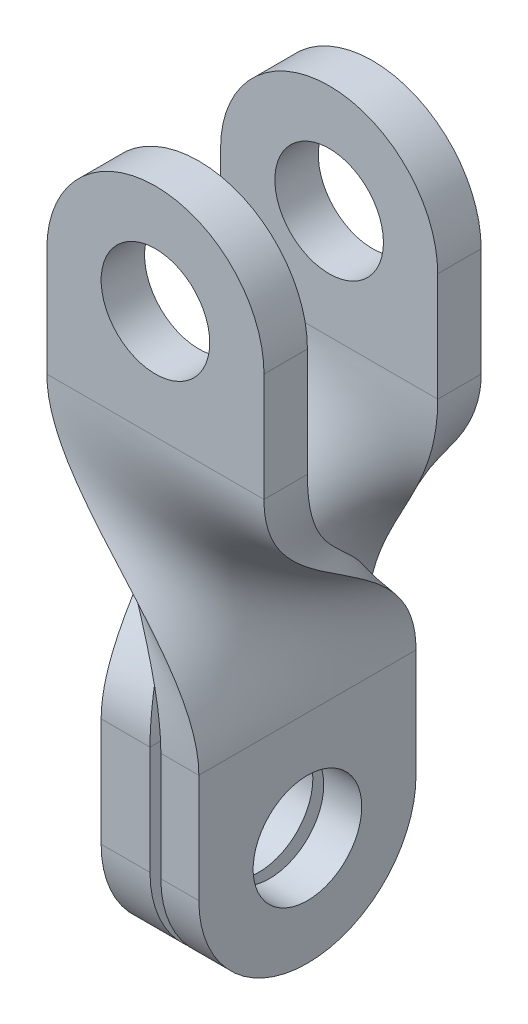
ISO-10303-21;
HEADER;
FILE_DESCRIPTION(('STEP AP214'),'2;1');
FILE_NAME('part.step','',(''),(''),'','','');
FILE_SCHEMA(('AUTOMOTIVE_DESIGN { 1 0 10303 214 1 1 1 1 }'));
ENDSEC;
DATA;
#1=APPLICATION_CONTEXT('core data for automotive mechanical design processes');
#2=APPLICATION_PROTOCOL_DEFINITION('international standard','automotive_design',2000,#1);
#3=PRODUCT_CONTEXT('',#1,'mechanical');
#4=PRODUCT('Part','Part','',(#3));
#5=PRODUCT_RELATED_PRODUCT_CATEGORY('part','',(#4));
#6=PRODUCT_DEFINITION_FORMATION('','',#4);
#7=PRODUCT_DEFINITION_CONTEXT('part definition',#1,'design');
#8=PRODUCT_DEFINITION('design','',#6,#7);
#9=PRODUCT_DEFINITION_SHAPE('','',#8);
#10=(LENGTH_UNIT() NAMED_UNIT(*) SI_UNIT(.MILLI.,.METRE.));
#11=(NAMED_UNIT(*) PLANE_ANGLE_UNIT() SI_UNIT($,.RADIAN.));
#12=(NAMED_UNIT(*) SI_UNIT($,.STERADIAN.) SOLID_ANGLE_UNIT());
#13=UNCERTAINTY_MEASURE_WITH_UNIT(LENGTH_MEASURE(1.E-05),#10,'distance_accuracy_value','');
#14=(GEOMETRIC_REPRESENTATION_CONTEXT(3) GLOBAL_UNCERTAINTY_ASSIGNED_CONTEXT((#13)) GLOBAL_UNIT_ASSIGNED_CONTEXT((#10,
#11,#12)) REPRESENTATION_CONTEXT('',''));
#15=CARTESIAN_POINT('',(0.,0.,0.));
#16=DIRECTION('',(0.,0.,1.));
#17=DIRECTION('',(1.,0.,0.));
#18=AXIS2_PLACEMENT_3D('',#15,#16,#17);
#19=CARTESIAN_POINT('',(-0.5,-4.5,1.));
#20=DIRECTION('',(0.,0.,-1.));
#21=DIRECTION('',(-1.,0.,0.));
#22=AXIS2_PLACEMENT_3D('',#19,#20,#21);
#23=PLANE('',#22);
#24=DIRECTION('',(0.,-1.,0.));
#25=VECTOR('',#24,1.);
#26=CARTESIAN_POINT('',(-0.05,-4.5,1.));
#27=LINE('',#26,#25);
#28=CARTESIAN_POINT('',(-0.05,-3.5,1.));
#29=VERTEX_POINT('',#28);
#30=CARTESIAN_POINT('',(-0.05,-4.5,1.));
#31=VERTEX_POINT('',#30);
#32=EDGE_CURVE('E577',#29,#31,#27,.T.);
#33=ORIENTED_EDGE('',*,*,#32,.F.);
#34=DIRECTION('',(1.,0.,0.));
#35=VECTOR('',#34,1.);
#36=CARTESIAN_POINT('',(-0.5,-3.5,1.));
#37=LINE('',#36,#35);
#38=CARTESIAN_POINT('',(-0.5,-3.5,1.));
#39=VERTEX_POINT('',#38);
#40=EDGE_CURVE('E604',#39,#29,#37,.T.);
#41=ORIENTED_EDGE('',*,*,#40,.F.);
#42=DIRECTION('',(0.,1.,0.));
#43=VECTOR('',#42,1.);
#44=CARTESIAN_POINT('',(-0.5,-4.5,1.));
#45=LINE('',#44,#43);
#46=CARTESIAN_POINT('',(-0.5,-4.5,1.));
#47=VERTEX_POINT('',#46);
#48=EDGE_CURVE('E598',#47,#39,#45,.T.);
#49=ORIENTED_EDGE('',*,*,#48,.F.);
#50=DIRECTION('',(1.,0.,0.));
#51=VECTOR('',#50,1.);
#52=CARTESIAN_POINT('',(-0.5,-4.5,1.));
#53=LINE('',#52,#51);
#54=EDGE_CURVE('E546',#47,#31,#53,.T.);
#55=ORIENTED_EDGE('',*,*,#54,.T.);
#56=EDGE_LOOP('',(#33,#41,#49,#55));
#57=FACE_BOUND('',#56,.T.);
#58=ADVANCED_FACE('F544',(#57),#23,.F.);
#59=CARTESIAN_POINT('',(-0.5,-3.5,1.));
#60=DIRECTION('',(0.,-1.,0.));
#61=DIRECTION('',(0.,0.,-1.));
#62=AXIS2_PLACEMENT_3D('',#59,#60,#61);
#63=PLANE('',#62);
#64=DIRECTION('',(0.,0.,1.));
#65=VECTOR('',#64,1.);
#66=CARTESIAN_POINT('',(-0.05,-3.5,1.));
#67=LINE('',#66,#65);
#68=CARTESIAN_POINT('',(-0.05,-3.5,-1.));
#69=VERTEX_POINT('',#68);
#70=EDGE_CURVE('E14',#69,#29,#67,.T.);
#71=ORIENTED_EDGE('',*,*,#70,.F.);
#72=DIRECTION('',(1.,0.,0.));
#73=VECTOR('',#72,1.);
#74=CARTESIAN_POINT('',(-0.5,-3.5,-1.));
#75=LINE('',#74,#73);
#76=CARTESIAN_POINT('',(-0.5,-3.5,-1.));
#77=VERTEX_POINT('',#76);
#78=EDGE_CURVE('E593',#77,#69,#75,.T.);
#79=ORIENTED_EDGE('',*,*,#78,.F.);
#80=DIRECTION('',(0.,0.,-1.));
#81=VECTOR('',#80,1.);
#82=CARTESIAN_POINT('',(-0.5,-3.5,1.));
#83=LINE('',#82,#81);
#84=EDGE_CURVE('E614',#39,#77,#83,.T.);
#85=ORIENTED_EDGE('',*,*,#84,.F.);
#86=ORIENTED_EDGE('',*,*,#40,.T.);
#87=EDGE_LOOP('',(#71,#79,#85,#86));
#88=FACE_BOUND('',#87,.T.);
#89=ADVANCED_FACE('F621',(#88),#63,.F.);
#90=CARTESIAN_POINT('',(-0.5,-3.5,-1.));
#91=DIRECTION('',(0.,0.,1.));
#92=DIRECTION('',(0.,-1.,0.));
#93=AXIS2_PLACEMENT_3D('',#90,#91,#92);
#94=PLANE('',#93);
#95=DIRECTION('',(0.,1.,0.));
#96=VECTOR('',#95,1.);
#97=CARTESIAN_POINT('',(-0.05,-3.5,-1.));
#98=LINE('',#97,#96);
#99=CARTESIAN_POINT('',(-0.05,-4.5,-1.));
#100=VERTEX_POINT('',#99);
#101=EDGE_CURVE('E552',#100,#69,#98,.T.);
#102=ORIENTED_EDGE('',*,*,#101,.F.);
#103=DIRECTION('',(1.,0.,0.));
#104=VECTOR('',#103,1.);
#105=CARTESIAN_POINT('',(-0.5,-4.5,-1.));
#106=LINE('',#105,#104);
#107=CARTESIAN_POINT('',(-0.5,-4.5,-1.));
#108=VERTEX_POINT('',#107);
#109=EDGE_CURVE('E591',#108,#100,#106,.T.);
#110=ORIENTED_EDGE('',*,*,#109,.F.);
#111=DIRECTION('',(0.,-1.,0.));
#112=VECTOR('',#111,1.);
#113=CARTESIAN_POINT('',(-0.5,-3.5,-1.));
#114=LINE('',#113,#112);
#115=EDGE_CURVE('E615',#77,#108,#114,.T.);
#116=ORIENTED_EDGE('',*,*,#115,.F.);
#117=ORIENTED_EDGE('',*,*,#78,.T.);
#118=EDGE_LOOP('',(#102,#110,#116,#117));
#119=FACE_BOUND('',#118,.T.);
#120=ADVANCED_FACE('F586',(#119),#94,.F.);
#121=CARTESIAN_POINT('',(-0.5,-4.5,0.));
#122=DIRECTION('',(1.,0.,0.));
#123=DIRECTION('',(0.,0.,-1.));
#124=AXIS2_PLACEMENT_3D('',#121,#122,#123);
#125=CYLINDRICAL_SURFACE('',#124,1.);
#126=CARTESIAN_POINT('',(-0.05,-4.5,0.));
#127=DIRECTION('',(1.,0.,0.));
#128=DIRECTION('',(0.,0.,1.));
#129=AXIS2_PLACEMENT_3D('',#126,#127,#128);
#130=CIRCLE('',#129,1.);
#131=EDGE_CURVE('E579',#31,#100,#130,.T.);
#132=ORIENTED_EDGE('',*,*,#131,.F.);
#133=ORIENTED_EDGE('',*,*,#54,.F.);
#134=CARTESIAN_POINT('',(-0.5,-4.5,0.));
#135=DIRECTION('',(-1.,0.,0.));
#136=DIRECTION('',(0.,0.,1.));
#137=AXIS2_PLACEMENT_3D('',#134,#135,#136);
#138=CIRCLE('',#137,1.);
#139=EDGE_CURVE('E600',#108,#47,#138,.T.);
#140=ORIENTED_EDGE('',*,*,#139,.F.);
#141=ORIENTED_EDGE('',*,*,#109,.T.);
#142=EDGE_LOOP('',(#132,#133,#140,#141));
#143=FACE_BOUND('',#142,.T.);
#144=ADVANCED_FACE('F597',(#143),#125,.T.);
#145=CARTESIAN_POINT('',(-0.5,-4.5,0.));
#146=DIRECTION('',(-1.,0.,0.));
#147=DIRECTION('',(0.,0.,1.));
#148=AXIS2_PLACEMENT_3D('',#145,#146,#147);
#149=PLANE('',#148);
#150=CARTESIAN_POINT('',(-0.5,-4.5,0.));
#151=DIRECTION('',(1.,0.,0.));
#152=DIRECTION('',(0.,0.,-1.));
#153=AXIS2_PLACEMENT_3D('',#150,#151,#152);
#154=CIRCLE('',#153,0.5);
#155=CARTESIAN_POINT('',(-0.5,-4.5,-0.5));
#156=VERTEX_POINT('',#155);
#157=EDGE_CURVE('E596',#156,#156,#154,.T.);
#158=ORIENTED_EDGE('',*,*,#157,.T.);
#159=EDGE_LOOP('',(#158));
#160=FACE_BOUND('',#159,.T.);
#161=ORIENTED_EDGE('',*,*,#48,.T.);
#162=ORIENTED_EDGE('',*,*,#84,.T.);
#163=ORIENTED_EDGE('',*,*,#115,.T.);
#164=ORIENTED_EDGE('',*,*,#139,.T.);
#165=EDGE_LOOP('',(#161,#162,#163,#164));
#166=FACE_BOUND('',#165,.T.);
#167=ADVANCED_FACE('F616',(#160,#166),#149,.T.);
#168=CARTESIAN_POINT('',(-0.5,-4.5,0.));
#169=DIRECTION('',(1.,0.,0.));
#170=DIRECTION('',(0.,0.,-1.));
#171=AXIS2_PLACEMENT_3D('',#168,#169,#170);
#172=CYLINDRICAL_SURFACE('',#171,0.5);
#173=CARTESIAN_POINT('',(-0.05,-4.5,0.));
#174=DIRECTION('',(1.,0.,0.));
#175=DIRECTION('',(0.,0.,-1.));
#176=AXIS2_PLACEMENT_3D('',#173,#174,#175);
#177=CIRCLE('',#176,0.5);
#178=CARTESIAN_POINT('',(-0.05,-4.5,-0.5));
#179=VERTEX_POINT('',#178);
#180=EDGE_CURVE('E609',#179,#179,#177,.T.);
#181=ORIENTED_EDGE('',*,*,#180,.T.);
#182=EDGE_LOOP('',(#181));
#183=FACE_BOUND('',#182,.T.);
#184=ORIENTED_EDGE('',*,*,#157,.F.);
#185=EDGE_LOOP('',(#184));
#186=FACE_BOUND('',#185,.T.);
#187=ADVANCED_FACE('F541',(#183,#186),#172,.F.);
#188=CARTESIAN_POINT('',(-0.05,-4.5,0.));
#189=DIRECTION('',(-1.,0.,0.));
#190=DIRECTION('',(0.,0.,1.));
#191=AXIS2_PLACEMENT_3D('',#188,#189,#190);
#192=PLANE('',#191);
#193=ORIENTED_EDGE('',*,*,#180,.F.);
#194=EDGE_LOOP('',(#193));
#195=FACE_BOUND('',#194,.T.);
#196=ORIENTED_EDGE('',*,*,#32,.T.);
#197=ORIENTED_EDGE('',*,*,#131,.T.);
#198=ORIENTED_EDGE('',*,*,#101,.T.);
#199=ORIENTED_EDGE('',*,*,#70,.T.);
#200=EDGE_LOOP('',(#196,#197,#198,#199));
#201=FACE_BOUND('',#200,.T.);
#202=ADVANCED_FACE('F578',(#195,#201),#192,.F.);
#203=CLOSED_SHELL('',(#58,#89,#120,#144,#167,#187,#202));
#204=MANIFOLD_SOLID_BREP('B2',#203);
#205=CARTESIAN_POINT('',(-1.,-1.,1.));
#206=DIRECTION('',(1.,0.,0.));
#207=DIRECTION('',(0.,0.,-1.));
#208=AXIS2_PLACEMENT_3D('',#205,#206,#207);
#209=PLANE('',#208);
#210=DIRECTION('',(0.,-1.,0.));
#211=VECTOR('',#210,1.);
#212=CARTESIAN_POINT('',(-1.,-1.,-0.6));
#213=LINE('',#212,#211);
#214=CARTESIAN_POINT('',(-1.,0.,-0.6));
#215=VERTEX_POINT('',#214);
#216=CARTESIAN_POINT('',(-1.,-1.,-0.6));
#217=VERTEX_POINT('',#216);
#218=EDGE_CURVE('E1003',#215,#217,#213,.T.);
#219=ORIENTED_EDGE('',*,*,#218,.F.);
#220=DIRECTION('',(0.,0.,-1.));
#221=VECTOR('',#220,1.);
#222=CARTESIAN_POINT('',(-1.,0.,1.));
#223=LINE('',#222,#221);
#224=CARTESIAN_POINT('',(-1.,0.,-1.));
#225=VERTEX_POINT('',#224);
#226=EDGE_CURVE('E996',#215,#225,#223,.T.);
#227=ORIENTED_EDGE('',*,*,#226,.T.);
#228=DIRECTION('',(0.,-1.,0.));
#229=VECTOR('',#228,1.);
#230=CARTESIAN_POINT('',(-1.,-1.,-1.));
#231=LINE('',#230,#229);
#232=CARTESIAN_POINT('',(-1.,-1.,-1.));
#233=VERTEX_POINT('',#232);
#234=EDGE_CURVE('E1004',#225,#233,#231,.T.);
#235=ORIENTED_EDGE('',*,*,#234,.T.);
#236=DIRECTION('',(0.,0.,-1.));
#237=VECTOR('',#236,1.);
#238=CARTESIAN_POINT('',(-1.,-1.,1.));
#239=LINE('',#238,#237);
#240=EDGE_CURVE('E951',#217,#233,#239,.T.);
#241=ORIENTED_EDGE('',*,*,#240,.F.);
#242=EDGE_LOOP('',(#219,#227,#235,#241));
#243=FACE_BOUND('',#242,.T.);
#244=ADVANCED_FACE('F950',(#243),#209,.F.);
#245=CARTESIAN_POINT('',(1.,0.,1.));
#246=DIRECTION('',(-1.,0.,0.));
#247=DIRECTION('',(0.,0.,1.));
#248=AXIS2_PLACEMENT_3D('',#245,#246,#247);
#249=PLANE('',#248);
#250=DIRECTION('',(0.,1.,0.));
#251=VECTOR('',#250,1.);
#252=CARTESIAN_POINT('',(1.,0.,-0.6));
#253=LINE('',#252,#251);
#254=CARTESIAN_POINT('',(1.,-1.,-0.6));
#255=VERTEX_POINT('',#254);
#256=CARTESIAN_POINT('',(1.,0.,-0.6));
#257=VERTEX_POINT('',#256);
#258=EDGE_CURVE('E960',#255,#257,#253,.T.);
#259=ORIENTED_EDGE('',*,*,#258,.F.);
#260=DIRECTION('',(0.,0.,1.));
#261=VECTOR('',#260,1.);
#262=CARTESIAN_POINT('',(1.,-1.,1.));
#263=LINE('',#262,#261);
#264=CARTESIAN_POINT('',(1.,-1.,-1.));
#265=VERTEX_POINT('',#264);
#266=EDGE_CURVE('E1028',#255,#265,#263,.F.);
#267=ORIENTED_EDGE('',*,*,#266,.T.);
#268=DIRECTION('',(0.,1.,0.));
#269=VECTOR('',#268,1.);
#270=CARTESIAN_POINT('',(1.,0.,-1.));
#271=LINE('',#270,#269);
#272=CARTESIAN_POINT('',(1.,0.,-1.));
#273=VERTEX_POINT('',#272);
#274=EDGE_CURVE('E1032',#265,#273,#271,.T.);
#275=ORIENTED_EDGE('',*,*,#274,.T.);
#276=DIRECTION('',(0.,0.,-1.));
#277=VECTOR('',#276,1.);
#278=CARTESIAN_POINT('',(1.,0.,1.));
#279=LINE('',#278,#277);
#280=EDGE_CURVE('E1011',#257,#273,#279,.T.);
#281=ORIENTED_EDGE('',*,*,#280,.F.);
#282=EDGE_LOOP('',(#259,#267,#275,#281));
#283=FACE_BOUND('',#282,.T.);
#284=ADVANCED_FACE('F1044',(#283),#249,.F.);
#285=CARTESIAN_POINT('',(0.,0.,1.));
#286=DIRECTION('',(0.,0.,-1.));
#287=DIRECTION('',(-1.,0.,0.));
#288=AXIS2_PLACEMENT_3D('',#285,#286,#287);
#289=CYLINDRICAL_SURFACE('',#288,1.);
#290=CARTESIAN_POINT('',(0.,0.,-0.6));
#291=DIRECTION('',(0.,0.,1.));
#292=DIRECTION('',(-1.,0.,0.));
#293=AXIS2_PLACEMENT_3D('',#290,#291,#292);
#294=CIRCLE('',#293,1.);
#295=EDGE_CURVE('E536',#257,#215,#294,.T.);
#296=ORIENTED_EDGE('',*,*,#295,.F.);
#297=ORIENTED_EDGE('',*,*,#280,.T.);
#298=CARTESIAN_POINT('',(0.,0.,-1.));
#299=DIRECTION('',(0.,0.,1.));
#300=DIRECTION('',(-1.,0.,0.));
#301=AXIS2_PLACEMENT_3D('',#298,#299,#300);
#302=CIRCLE('',#301,1.);
#303=EDGE_CURVE('E1009',#273,#225,#302,.T.);
#304=ORIENTED_EDGE('',*,*,#303,.T.);
#305=ORIENTED_EDGE('',*,*,#226,.F.);
#306=EDGE_LOOP('',(#296,#297,#304,#305));
#307=FACE_BOUND('',#306,.T.);
#308=ADVANCED_FACE('F1013',(#307),#289,.T.);
#309=CARTESIAN_POINT('',(0.,0.,-1.));
#310=DIRECTION('',(0.,0.,-1.));
#311=DIRECTION('',(-1.,0.,0.));
#312=AXIS2_PLACEMENT_3D('',#309,#310,#311);
#313=PLANE('',#312);
#314=ORIENTED_EDGE('',*,*,#234,.F.);
#315=ORIENTED_EDGE('',*,*,#303,.F.);
#316=ORIENTED_EDGE('',*,*,#274,.F.);
#317=DIRECTION('',(-1.,0.,0.));
#318=VECTOR('',#317,1.);
#319=CARTESIAN_POINT('',(0.,-1.,-1.));
#320=LINE('',#319,#318);
#321=EDGE_CURVE('E1023',#233,#265,#320,.F.);
#322=ORIENTED_EDGE('',*,*,#321,.F.);
#323=EDGE_LOOP('',(#314,#315,#316,#322));
#324=FACE_BOUND('',#323,.T.);
#325=CARTESIAN_POINT('',(0.,0.,-1.));
#326=DIRECTION('',(0.,0.,1.));
#327=DIRECTION('',(1.,0.,0.));
#328=AXIS2_PLACEMENT_3D('',#325,#326,#327);
#329=CIRCLE('',#328,0.5);
#330=CARTESIAN_POINT('',(0.5,0.,-1.));
#331=VERTEX_POINT('',#330);
#332=EDGE_CURVE('E1020',#331,#331,#329,.T.);
#333=ORIENTED_EDGE('',*,*,#332,.T.);
#334=EDGE_LOOP('',(#333));
#335=FACE_BOUND('',#334,.T.);
#336=ADVANCED_FACE('F1019',(#324,#335),#313,.T.);
#337=CARTESIAN_POINT('',(0.,0.,1.));
#338=DIRECTION('',(0.,0.,-1.));
#339=DIRECTION('',(-1.,0.,0.));
#340=AXIS2_PLACEMENT_3D('',#337,#338,#339);
#341=CYLINDRICAL_SURFACE('',#340,0.5);
#342=CARTESIAN_POINT('',(0.,0.,-0.6));
#343=DIRECTION('',(0.,0.,1.));
#344=DIRECTION('',(1.,0.,0.));
#345=AXIS2_PLACEMENT_3D('',#342,#343,#344);
#346=CIRCLE('',#345,0.5);
#347=CARTESIAN_POINT('',(0.5,0.,-0.6));
#348=VERTEX_POINT('',#347);
#349=EDGE_CURVE('E1049',#348,#348,#346,.T.);
#350=ORIENTED_EDGE('',*,*,#349,.T.);
#351=EDGE_LOOP('',(#350));
#352=FACE_BOUND('',#351,.T.);
#353=ORIENTED_EDGE('',*,*,#332,.F.);
#354=EDGE_LOOP('',(#353));
#355=FACE_BOUND('',#354,.T.);
#356=ADVANCED_FACE('F949',(#352,#355),#341,.F.);
#357=CARTESIAN_POINT('',(0.,0.,-0.6));
#358=DIRECTION('',(0.,0.,-1.));
#359=DIRECTION('',(-1.,0.,0.));
#360=AXIS2_PLACEMENT_3D('',#357,#358,#359);
#361=PLANE('',#360);
#362=ORIENTED_EDGE('',*,*,#349,.F.);
#363=EDGE_LOOP('',(#362));
#364=FACE_BOUND('',#363,.T.);
#365=ORIENTED_EDGE('',*,*,#218,.T.);
#366=DIRECTION('',(-1.,0.,0.));
#367=VECTOR('',#366,1.);
#368=CARTESIAN_POINT('',(0.,-1.,-0.6));
#369=LINE('',#368,#367);
#370=EDGE_CURVE('E984',#217,#255,#369,.F.);
#371=ORIENTED_EDGE('',*,*,#370,.T.);
#372=ORIENTED_EDGE('',*,*,#258,.T.);
#373=ORIENTED_EDGE('',*,*,#295,.T.);
#374=EDGE_LOOP('',(#365,#371,#372,#373));
#375=FACE_BOUND('',#374,.T.);
#376=ADVANCED_FACE('F1047',(#364,#375),#361,.F.);
#377=CARTESIAN_POINT('',(-0.5,-3.5,1.));
#378=DIRECTION('',(0.,-1.,0.));
#379=DIRECTION('',(0.,0.,-1.));
#380=AXIS2_PLACEMENT_3D('',#377,#378,#379);
#381=PLANE('',#380);
#382=DIRECTION('',(0.,0.,1.));
#383=VECTOR('',#382,1.);
#384=CARTESIAN_POINT('',(-0.05,-3.5,1.));
#385=LINE('',#384,#383);
#386=CARTESIAN_POINT('',(-0.05,-3.5,-1.));
#387=VERTEX_POINT('',#386);
#388=CARTESIAN_POINT('',(-0.05,-3.5,1.));
#389=VERTEX_POINT('',#388);
#390=EDGE_CURVE('E1072',#387,#389,#385,.T.);
#391=ORIENTED_EDGE('',*,*,#390,.T.);
#392=DIRECTION('',(1.,0.,0.));
#393=VECTOR('',#392,1.);
#394=CARTESIAN_POINT('',(-0.5,-3.5,1.));
#395=LINE('',#394,#393);
#396=CARTESIAN_POINT('',(-0.5,-3.5,1.));
#397=VERTEX_POINT('',#396);
#398=EDGE_CURVE('E1052',#397,#389,#395,.T.);
#399=ORIENTED_EDGE('',*,*,#398,.F.);
#400=DIRECTION('',(0.,0.,-1.));
#401=VECTOR('',#400,1.);
#402=CARTESIAN_POINT('',(-0.5,-3.5,1.));
#403=LINE('',#402,#401);
#404=CARTESIAN_POINT('',(-0.5,-3.5,-1.));
#405=VERTEX_POINT('',#404);
#406=EDGE_CURVE('E1128',#397,#405,#403,.T.);
#407=ORIENTED_EDGE('',*,*,#406,.T.);
#408=DIRECTION('',(1.,0.,0.));
#409=VECTOR('',#408,1.);
#410=CARTESIAN_POINT('',(-0.5,-3.5,-1.));
#411=LINE('',#410,#409);
#412=EDGE_CURVE('E1164',#405,#387,#411,.T.);
#413=ORIENTED_EDGE('',*,*,#412,.T.);
#414=EDGE_LOOP('',(#391,#399,#407,#413));
#415=FACE_BOUND('',#414,.T.);
#416=ADVANCED_FACE('F1141',(#415),#381,.T.);
#417=CARTESIAN_POINT('',(-0.5,-3.5,1.));
#418=CARTESIAN_POINT('',(-0.5,-2.51859259682588,1.));
#419=CARTESIAN_POINT('',(-1.,-1.98140740317412,-1.));
#420=CARTESIAN_POINT('',(-1.,-1.,-1.));
#421=CARTESIAN_POINT('',(-0.425,-3.5,1.));
#422=CARTESIAN_POINT('',(-0.425,-2.5240902102044,1.));
#423=CARTESIAN_POINT('',(-1.,-1.9759097897956,-0.933333333333333));
#424=CARTESIAN_POINT('',(-1.,-1.,-0.933333333333333));
#425=CARTESIAN_POINT('',(-0.275,-3.5,1.));
#426=CARTESIAN_POINT('',(-0.275,-2.53508543696142,1.));
#427=CARTESIAN_POINT('',(-1.,-1.96491456303857,-0.8));
#428=CARTESIAN_POINT('',(-1.,-1.,-0.8));
#429=CARTESIAN_POINT('',(-0.125,-3.5,1.));
#430=CARTESIAN_POINT('',(-0.125,-2.54060780230499,1.));
#431=CARTESIAN_POINT('',(-1.,-1.95939219769501,-0.666666666666667));
#432=CARTESIAN_POINT('',(-1.,-1.,-0.666666666666667));
#433=CARTESIAN_POINT('',(-0.05,-3.5,1.));
#434=CARTESIAN_POINT('',(-0.05,-2.54336898497677,1.));
#435=CARTESIAN_POINT('',(-1.,-1.95663101502323,-0.6));
#436=CARTESIAN_POINT('',(-1.,-1.,-0.6));
#437=B_SPLINE_SURFACE_WITH_KNOTS('',3,3,((#417,#418,#419,#420),(#421,#422,#423,#424),(#425,#426,
#427,#428),(#429,#430,#431,#432),(#433,#434,#435,#436)),.UNSPECIFIED.,.F.,.F.,.F.,(4,1,4),(4,4),
(0.,0.5,1.),(0.,1.),.UNSPECIFIED.);
#438=CARTESIAN_POINT('',(-0.05,-3.5,1.));
#439=CARTESIAN_POINT('',(-0.05,-2.54336898497677,1.));
#440=CARTESIAN_POINT('',(-1.,-1.95663101502323,-0.6));
#441=CARTESIAN_POINT('',(-1.,-1.,-0.6));
#442=B_SPLINE_CURVE_WITH_KNOTS('',3,(#438,#439,#440,#441),.UNSPECIFIED.,.F.,.F.,(4,4),(0.,1.),.UNSPECIFIED.);
#443=EDGE_CURVE('E989',#389,#217,#442,.T.);
#444=CARTESIAN_POINT('',(-0.5,-3.5,1.));
#445=CARTESIAN_POINT('',(-0.5,-2.51859259682588,1.));
#446=CARTESIAN_POINT('',(-1.,-1.98140740317412,-1.));
#447=CARTESIAN_POINT('',(-1.,-1.,-1.));
#448=B_SPLINE_CURVE_WITH_KNOTS('',3,(#444,#445,#446,#447),.UNSPECIFIED.,.F.,.F.,(4,4),(0.,1.),.UNSPECIFIED.);
#449=EDGE_CURVE('E1037',#233,#397,#448,.F.);
#450=ORIENTED_EDGE('',*,*,#398,.T.);
#451=ORIENTED_EDGE('',*,*,#443,.T.);
#452=ORIENTED_EDGE('',*,*,#240,.T.);
#453=ORIENTED_EDGE('',*,*,#449,.T.);
#454=EDGE_LOOP('',(#450,#451,#452,#453));
#455=FACE_BOUND('',#454,.T.);
#456=ADVANCED_FACE('F1050',(#455),#437,.T.);
#457=CARTESIAN_POINT('',(-0.05,-3.5,1.));
#458=CARTESIAN_POINT('',(-0.05,-2.54336898497677,1.));
#459=CARTESIAN_POINT('',(-1.,-1.95663101502323,-0.6));
#460=CARTESIAN_POINT('',(-1.,-1.,-0.6));
#461=CARTESIAN_POINT('',(-0.05,-3.5,0.666666666666667));
#462=CARTESIAN_POINT('',(-0.05,-2.5916101018473,0.666666666666667));
#463=CARTESIAN_POINT('',(-0.666666666666667,-1.9083898981527,-0.6));
#464=CARTESIAN_POINT('',(-0.666666666666667,-1.,-0.6));
#465=CARTESIAN_POINT('',(-0.05,-3.5,0.));
#466=CARTESIAN_POINT('',(-0.05,-2.68809233558837,0.));
#467=CARTESIAN_POINT('',(0.,-1.81190766441163,-0.6));
#468=CARTESIAN_POINT('',(0.,-1.,-0.6));
#469=CARTESIAN_POINT('',(-0.05,-3.5,-0.666666666666666));
#470=CARTESIAN_POINT('',(-0.05,-2.64168935434281,-0.666666666666666));
#471=CARTESIAN_POINT('',(0.666666666666667,-1.85831064565718,-0.6));
#472=CARTESIAN_POINT('',(0.666666666666667,-1.,-0.6));
#473=CARTESIAN_POINT('',(-0.05,-3.5,-1.));
#474=CARTESIAN_POINT('',(-0.05,-2.61848786372004,-1.));
#475=CARTESIAN_POINT('',(1.,-1.88151213627996,-0.6));
#476=CARTESIAN_POINT('',(1.,-1.,-0.6));
#477=B_SPLINE_SURFACE_WITH_KNOTS('',3,3,((#457,#458,#459,#460),(#461,#462,#463,#464),(#465,#466,
#467,#468),(#469,#470,#471,#472),(#473,#474,#475,#476)),.UNSPECIFIED.,.F.,.F.,.F.,(4,1,4),(4,4),
(0.,0.5,1.),(0.,1.),.UNSPECIFIED.);
#478=CARTESIAN_POINT('',(-0.05,-3.5,-1.));
#479=CARTESIAN_POINT('',(-0.05,-2.61848786372004,-1.));
#480=CARTESIAN_POINT('',(1.,-1.88151213627996,-0.6));
#481=CARTESIAN_POINT('',(1.,-1.,-0.6));
#482=B_SPLINE_CURVE_WITH_KNOTS('',3,(#478,#479,#480,#481),.UNSPECIFIED.,.F.,.F.,(4,4),(0.,1.),.UNSPECIFIED.);
#483=EDGE_CURVE('E1054',#387,#255,#482,.T.);
#484=ORIENTED_EDGE('',*,*,#390,.F.);
#485=ORIENTED_EDGE('',*,*,#483,.T.);
#486=ORIENTED_EDGE('',*,*,#370,.F.);
#487=ORIENTED_EDGE('',*,*,#443,.F.);
#488=EDGE_LOOP('',(#484,#485,#486,#487));
#489=FACE_BOUND('',#488,.T.);
#490=ADVANCED_FACE('F1080',(#489),#477,.T.);
#491=CARTESIAN_POINT('',(-0.5,-3.5,-1.));
#492=CARTESIAN_POINT('',(-0.5,-2.58357147718214,-1.));
#493=CARTESIAN_POINT('',(1.,-1.91642852281786,-1.));
#494=CARTESIAN_POINT('',(1.,-1.,-1.));
#495=CARTESIAN_POINT('',(-0.5,-3.5,-0.666666666666666));
#496=CARTESIAN_POINT('',(-0.5,-2.60667269986817,-0.666666666666666));
#497=CARTESIAN_POINT('',(0.666666666666667,-1.89332730013183,-1.));
#498=CARTESIAN_POINT('',(0.666666666666667,-1.,-1.));
#499=CARTESIAN_POINT('',(-0.5,-3.5,0.));
#500=CARTESIAN_POINT('',(-0.5,-2.65287514524025,0.));
#501=CARTESIAN_POINT('',(0.,-1.84712485475975,-1.));
#502=CARTESIAN_POINT('',(0.,-1.,-1.));
#503=CARTESIAN_POINT('',(-0.5,-3.5,0.666666666666667));
#504=CARTESIAN_POINT('',(-0.5,-2.56335344629734,0.666666666666667));
#505=CARTESIAN_POINT('',(-0.666666666666667,-1.93664655370266,-1.));
#506=CARTESIAN_POINT('',(-0.666666666666667,-1.,-1.));
#507=CARTESIAN_POINT('',(-0.5,-3.5,1.));
#508=CARTESIAN_POINT('',(-0.5,-2.51859259682588,1.));
#509=CARTESIAN_POINT('',(-1.,-1.98140740317412,-1.));
#510=CARTESIAN_POINT('',(-1.,-1.,-1.));
#511=B_SPLINE_SURFACE_WITH_KNOTS('',3,3,((#491,#492,#493,#494),(#495,#496,#497,#498),(#499,#500,
#501,#502),(#503,#504,#505,#506),(#507,#508,#509,#510)),.UNSPECIFIED.,.F.,.F.,.F.,(4,1,4),(4,4),
(0.,0.5,1.),(0.,1.),.UNSPECIFIED.);
#512=CARTESIAN_POINT('',(-0.5,-3.5,-1.));
#513=CARTESIAN_POINT('',(-0.5,-2.58357147718214,-1.));
#514=CARTESIAN_POINT('',(1.,-1.91642852281786,-1.));
#515=CARTESIAN_POINT('',(1.,-1.,-1.));
#516=B_SPLINE_CURVE_WITH_KNOTS('',3,(#512,#513,#514,#515),.UNSPECIFIED.,.F.,.F.,(4,4),(0.,1.),.UNSPECIFIED.);
#517=EDGE_CURVE('E1008',#405,#265,#516,.T.);
#518=ORIENTED_EDGE('',*,*,#406,.F.);
#519=ORIENTED_EDGE('',*,*,#449,.F.);
#520=ORIENTED_EDGE('',*,*,#321,.T.);
#521=ORIENTED_EDGE('',*,*,#517,.F.);
#522=EDGE_LOOP('',(#518,#519,#520,#521));
#523=FACE_BOUND('',#522,.T.);
#524=ADVANCED_FACE('F1038',(#523),#511,.T.);
#525=CARTESIAN_POINT('',(-0.05,-3.5,-1.));
#526=CARTESIAN_POINT('',(-0.05,-2.61848786372004,-1.));
#527=CARTESIAN_POINT('',(1.,-1.88151213627996,-0.6));
#528=CARTESIAN_POINT('',(1.,-1.,-0.6));
#529=CARTESIAN_POINT('',(-0.125,-3.5,-1.));
#530=CARTESIAN_POINT('',(-0.125,-2.61413975864732,-1.));
#531=CARTESIAN_POINT('',(1.,-1.88586024135268,-0.666666666666667));
#532=CARTESIAN_POINT('',(1.,-1.,-0.666666666666667));
#533=CARTESIAN_POINT('',(-0.275,-3.5,-1.));
#534=CARTESIAN_POINT('',(-0.275,-2.60544354850189,-1.));
#535=CARTESIAN_POINT('',(1.,-1.89455645149811,-0.8));
#536=CARTESIAN_POINT('',(1.,-1.,-0.8));
#537=CARTESIAN_POINT('',(-0.425,-3.5,-1.));
#538=CARTESIAN_POINT('',(-0.425,-2.59086216762206,-1.));
#539=CARTESIAN_POINT('',(1.,-1.90913783237794,-0.933333333333333));
#540=CARTESIAN_POINT('',(1.,-1.,-0.933333333333333));
#541=CARTESIAN_POINT('',(-0.5,-3.5,-1.));
#542=CARTESIAN_POINT('',(-0.5,-2.58357147718214,-1.));
#543=CARTESIAN_POINT('',(1.,-1.91642852281786,-1.));
#544=CARTESIAN_POINT('',(1.,-1.,-1.));
#545=B_SPLINE_SURFACE_WITH_KNOTS('',3,3,((#525,#526,#527,#528),(#529,#530,#531,#532),(#533,#534,
#535,#536),(#537,#538,#539,#540),(#541,#542,#543,#544)),.UNSPECIFIED.,.F.,.F.,.F.,(4,1,4),(4,4),
(0.,0.5,1.),(0.,1.),.UNSPECIFIED.);
#546=ORIENTED_EDGE('',*,*,#412,.F.);
#547=ORIENTED_EDGE('',*,*,#517,.T.);
#548=ORIENTED_EDGE('',*,*,#266,.F.);
#549=ORIENTED_EDGE('',*,*,#483,.F.);
#550=EDGE_LOOP('',(#546,#547,#548,#549));
#551=FACE_BOUND('',#550,.T.);
#552=ADVANCED_FACE('F1102',(#551),#545,.T.);
#553=CLOSED_SHELL('',(#244,#284,#308,#336,#356,#376,#416,#456,#490,#524,#552));
#554=MANIFOLD_SOLID_BREP('B8',#553);
#555=CARTESIAN_POINT('',(0.,0.,1.));
#556=DIRECTION('',(0.,0.,-1.));
#557=DIRECTION('',(-1.,0.,0.));
#558=AXIS2_PLACEMENT_3D('',#555,#556,#557);
#559=CYLINDRICAL_SURFACE('',#558,1.);
#560=DIRECTION('',(0.,0.,-1.));
#561=VECTOR('',#560,1.);
#562=CARTESIAN_POINT('',(1.,0.,1.));
#563=LINE('',#562,#561);
#564=CARTESIAN_POINT('',(1.,0.,1.));
#565=VERTEX_POINT('',#564);
#566=CARTESIAN_POINT('',(1.,0.,0.6));
#567=VERTEX_POINT('',#566);
#568=EDGE_CURVE('E1639',#565,#567,#563,.T.);
#569=ORIENTED_EDGE('',*,*,#568,.T.);
#570=CARTESIAN_POINT('',(0.,0.,0.6));
#571=DIRECTION('',(0.,0.,1.));
#572=DIRECTION('',(-1.,0.,0.));
#573=AXIS2_PLACEMENT_3D('',#570,#571,#572);
#574=CIRCLE('',#573,1.);
#575=CARTESIAN_POINT('',(-1.,0.,0.6));
#576=VERTEX_POINT('',#575);
#577=EDGE_CURVE('E1660',#567,#576,#574,.T.);
#578=ORIENTED_EDGE('',*,*,#577,.T.);
#579=DIRECTION('',(0.,0.,-1.));
#580=VECTOR('',#579,1.);
#581=CARTESIAN_POINT('',(-1.,0.,1.));
#582=LINE('',#581,#580);
#583=CARTESIAN_POINT('',(-1.,0.,1.));
#584=VERTEX_POINT('',#583);
#585=EDGE_CURVE('E1645',#584,#576,#582,.T.);
#586=ORIENTED_EDGE('',*,*,#585,.F.);
#587=CARTESIAN_POINT('',(0.,0.,1.));
#588=DIRECTION('',(0.,0.,1.));
#589=DIRECTION('',(-1.,0.,0.));
#590=AXIS2_PLACEMENT_3D('',#587,#588,#589);
#591=CIRCLE('',#590,1.);
#592=EDGE_CURVE('E1628',#565,#584,#591,.T.);
#593=ORIENTED_EDGE('',*,*,#592,.F.);
#594=EDGE_LOOP('',(#569,#578,#586,#593));
#595=FACE_BOUND('',#594,.T.);
#596=ADVANCED_FACE('F1563',(#595),#559,.T.);
#597=CARTESIAN_POINT('',(1.,0.,1.));
#598=DIRECTION('',(-1.,0.,0.));
#599=DIRECTION('',(0.,0.,1.));
#600=AXIS2_PLACEMENT_3D('',#597,#598,#599);
#601=PLANE('',#600);
#602=DIRECTION('',(0.,0.,1.));
#603=VECTOR('',#602,1.);
#604=CARTESIAN_POINT('',(1.,-1.,1.));
#605=LINE('',#604,#603);
#606=CARTESIAN_POINT('',(1.,-1.,1.));
#607=VERTEX_POINT('',#606);
#608=CARTESIAN_POINT('',(1.,-1.,0.6));
#609=VERTEX_POINT('',#608);
#610=EDGE_CURVE('E1579',#607,#609,#605,.F.);
#611=ORIENTED_EDGE('',*,*,#610,.T.);
#612=DIRECTION('',(0.,1.,0.));
#613=VECTOR('',#612,1.);
#614=CARTESIAN_POINT('',(1.,0.,0.6));
#615=LINE('',#614,#613);
#616=EDGE_CURVE('E1644',#609,#567,#615,.T.);
#617=ORIENTED_EDGE('',*,*,#616,.T.);
#618=ORIENTED_EDGE('',*,*,#568,.F.);
#619=DIRECTION('',(0.,1.,0.));
#620=VECTOR('',#619,1.);
#621=CARTESIAN_POINT('',(1.,0.,1.));
#622=LINE('',#621,#620);
#623=EDGE_CURVE('E1625',#607,#565,#622,.T.);
#624=ORIENTED_EDGE('',*,*,#623,.F.);
#625=EDGE_LOOP('',(#611,#617,#618,#624));
#626=FACE_BOUND('',#625,.T.);
#627=ADVANCED_FACE('F1638',(#626),#601,.F.);
#628=CARTESIAN_POINT('',(-1.,-1.,1.));
#629=DIRECTION('',(1.,0.,0.));
#630=DIRECTION('',(0.,0.,-1.));
#631=AXIS2_PLACEMENT_3D('',#628,#629,#630);
#632=PLANE('',#631);
#633=ORIENTED_EDGE('',*,*,#585,.T.);
#634=DIRECTION('',(0.,-1.,0.));
#635=VECTOR('',#634,1.);
#636=CARTESIAN_POINT('',(-1.,-1.,0.6));
#637=LINE('',#636,#635);
#638=CARTESIAN_POINT('',(-1.,-1.,0.6));
#639=VERTEX_POINT('',#638);
#640=EDGE_CURVE('E1586',#576,#639,#637,.T.);
#641=ORIENTED_EDGE('',*,*,#640,.T.);
#642=DIRECTION('',(0.,0.,-1.));
#643=VECTOR('',#642,1.);
#644=CARTESIAN_POINT('',(-1.,-1.,1.));
#645=LINE('',#644,#643);
#646=CARTESIAN_POINT('',(-1.,-1.,1.));
#647=VERTEX_POINT('',#646);
#648=EDGE_CURVE('E944',#647,#639,#645,.T.);
#649=ORIENTED_EDGE('',*,*,#648,.F.);
#650=DIRECTION('',(0.,-1.,0.));
#651=VECTOR('',#650,1.);
#652=CARTESIAN_POINT('',(-1.,-1.,1.));
#653=LINE('',#652,#651);
#654=EDGE_CURVE('E1653',#584,#647,#653,.T.);
#655=ORIENTED_EDGE('',*,*,#654,.F.);
#656=EDGE_LOOP('',(#633,#641,#649,#655));
#657=FACE_BOUND('',#656,.T.);
#658=ADVANCED_FACE('F1567',(#657),#632,.F.);
#659=CARTESIAN_POINT('',(0.,0.,1.));
#660=DIRECTION('',(0.,0.,-1.));
#661=DIRECTION('',(-1.,0.,0.));
#662=AXIS2_PLACEMENT_3D('',#659,#660,#661);
#663=PLANE('',#662);
#664=ORIENTED_EDGE('',*,*,#654,.T.);
#665=DIRECTION('',(-1.,0.,0.));
#666=VECTOR('',#665,1.);
#667=CARTESIAN_POINT('',(0.,-1.,1.));
#668=LINE('',#667,#666);
#669=EDGE_CURVE('E1634',#647,#607,#668,.F.);
#670=ORIENTED_EDGE('',*,*,#669,.T.);
#671=ORIENTED_EDGE('',*,*,#623,.T.);
#672=ORIENTED_EDGE('',*,*,#592,.T.);
#673=EDGE_LOOP('',(#664,#670,#671,#672));
#674=FACE_BOUND('',#673,.T.);
#675=CARTESIAN_POINT('',(0.,0.,1.));
#676=DIRECTION('',(0.,0.,1.));
#677=DIRECTION('',(1.,0.,0.));
#678=AXIS2_PLACEMENT_3D('',#675,#676,#677);
#679=CIRCLE('',#678,0.5);
#680=CARTESIAN_POINT('',(0.5,0.,1.));
#681=VERTEX_POINT('',#680);
#682=EDGE_CURVE('E1651',#681,#681,#679,.T.);
#683=ORIENTED_EDGE('',*,*,#682,.F.);
#684=EDGE_LOOP('',(#683));
#685=FACE_BOUND('',#684,.T.);
#686=ADVANCED_FACE('F1629',(#674,#685),#663,.F.);
#687=CARTESIAN_POINT('',(0.,0.,1.));
#688=DIRECTION('',(0.,0.,-1.));
#689=DIRECTION('',(-1.,0.,0.));
#690=AXIS2_PLACEMENT_3D('',#687,#688,#689);
#691=CYLINDRICAL_SURFACE('',#690,0.5);
#692=ORIENTED_EDGE('',*,*,#682,.T.);
#693=EDGE_LOOP('',(#692));
#694=FACE_BOUND('',#693,.T.);
#695=CARTESIAN_POINT('',(0.,0.,0.6));
#696=DIRECTION('',(0.,0.,1.));
#697=DIRECTION('',(1.,0.,0.));
#698=AXIS2_PLACEMENT_3D('',#695,#696,#697);
#699=CIRCLE('',#698,0.5);
#700=CARTESIAN_POINT('',(0.5,0.,0.6));
#701=VERTEX_POINT('',#700);
#702=EDGE_CURVE('E1656',#701,#701,#699,.T.);
#703=ORIENTED_EDGE('',*,*,#702,.F.);
#704=EDGE_LOOP('',(#703));
#705=FACE_BOUND('',#704,.T.);
#706=ADVANCED_FACE('F1962',(#694,#705),#691,.F.);
#707=CARTESIAN_POINT('',(0.,0.,0.6));
#708=DIRECTION('',(0.,0.,-1.));
#709=DIRECTION('',(-1.,0.,0.));
#710=AXIS2_PLACEMENT_3D('',#707,#708,#709);
#711=PLANE('',#710);
#712=ORIENTED_EDGE('',*,*,#702,.T.);
#713=EDGE_LOOP('',(#712));
#714=FACE_BOUND('',#713,.T.);
#715=ORIENTED_EDGE('',*,*,#640,.F.);
#716=ORIENTED_EDGE('',*,*,#577,.F.);
#717=ORIENTED_EDGE('',*,*,#616,.F.);
#718=DIRECTION('',(-1.,0.,0.));
#719=VECTOR('',#718,1.);
#720=CARTESIAN_POINT('',(0.,-1.,0.6));
#721=LINE('',#720,#719);
#722=EDGE_CURVE('E1657',#639,#609,#721,.F.);
#723=ORIENTED_EDGE('',*,*,#722,.F.);
#724=EDGE_LOOP('',(#715,#716,#717,#723));
#725=FACE_BOUND('',#724,.T.);
#726=ADVANCED_FACE('F1782',(#714,#725),#711,.T.);
#727=CARTESIAN_POINT('',(0.4,-3.5,-1.));
#728=CARTESIAN_POINT('',(0.4,-2.51520676767057,-1.));
#729=CARTESIAN_POINT('',(1.,-1.98479323232943,1.));
#730=CARTESIAN_POINT('',(1.,-1.,1.));
#731=CARTESIAN_POINT('',(0.341666666666667,-3.5,-1.));
#732=CARTESIAN_POINT('',(0.341666666666667,-2.52093242444731,-1.));
#733=CARTESIAN_POINT('',(1.,-1.97906757555269,0.933333333333333));
#734=CARTESIAN_POINT('',(1.,-1.,0.933333333333333));
#735=CARTESIAN_POINT('',(0.225,-3.5,-1.));
#736=CARTESIAN_POINT('',(0.225,-2.53238373800079,-1.));
#737=CARTESIAN_POINT('',(1.,-1.96761626199921,0.8));
#738=CARTESIAN_POINT('',(1.,-1.,0.8));
#739=CARTESIAN_POINT('',(0.108333333333333,-3.5,-1.));
#740=CARTESIAN_POINT('',(0.108333333333333,-2.53970723598478,-1.));
#741=CARTESIAN_POINT('',(1.,-1.96029276401522,0.666666666666667));
#742=CARTESIAN_POINT('',(1.,-1.,0.666666666666667));
#743=CARTESIAN_POINT('',(0.05,-3.5,-1.));
#744=CARTESIAN_POINT('',(0.05,-2.54336898497677,-1.));
#745=CARTESIAN_POINT('',(1.,-1.95663101502323,0.6));
#746=CARTESIAN_POINT('',(1.,-1.,0.6));
#747=B_SPLINE_SURFACE_WITH_KNOTS('',3,3,((#727,#728,#729,#730),(#731,#732,#733,#734),(#735,#736,
#737,#738),(#739,#740,#741,#742),(#743,#744,#745,#746)),.UNSPECIFIED.,.F.,.F.,.F.,(4,1,4),(4,4),
(0.,0.5,1.),(0.,1.),.UNSPECIFIED.);
#748=DIRECTION('',(1.,0.,0.));
#749=VECTOR('',#748,1.);
#750=CARTESIAN_POINT('',(-0.5,-3.5,-1.));
#751=LINE('',#750,#749);
#752=CARTESIAN_POINT('',(0.05,-3.5,-1.));
#753=VERTEX_POINT('',#752);
#754=CARTESIAN_POINT('',(0.4,-3.5,-1.));
#755=VERTEX_POINT('',#754);
#756=EDGE_CURVE('E1731',#753,#755,#751,.T.);
#757=CARTESIAN_POINT('',(0.05,-3.5,-1.));
#758=CARTESIAN_POINT('',(0.05,-2.54336898497677,-1.));
#759=CARTESIAN_POINT('',(1.,-1.95663101502323,0.6));
#760=CARTESIAN_POINT('',(1.,-1.,0.6));
#761=B_SPLINE_CURVE_WITH_KNOTS('',3,(#757,#758,#759,#760),.UNSPECIFIED.,.F.,.F.,(4,4),(0.,1.),.UNSPECIFIED.);
#762=EDGE_CURVE('E1797',#753,#609,#761,.T.);
#763=CARTESIAN_POINT('',(0.4,-3.5,-1.));
#764=CARTESIAN_POINT('',(0.4,-2.51520676767057,-1.));
#765=CARTESIAN_POINT('',(1.,-1.98479323232943,1.));
#766=CARTESIAN_POINT('',(1.,-1.,1.));
#767=B_SPLINE_CURVE_WITH_KNOTS('',3,(#763,#764,#765,#766),.UNSPECIFIED.,.F.,.F.,(4,4),(0.,1.),.UNSPECIFIED.);
#768=EDGE_CURVE('E1728',#607,#755,#767,.F.);
#769=ORIENTED_EDGE('',*,*,#756,.F.);
#770=ORIENTED_EDGE('',*,*,#762,.T.);
#771=ORIENTED_EDGE('',*,*,#610,.F.);
#772=ORIENTED_EDGE('',*,*,#768,.T.);
#773=EDGE_LOOP('',(#769,#770,#771,#772));
#774=FACE_BOUND('',#773,.T.);
#775=ADVANCED_FACE('F1766',(#774),#747,.T.);
#776=CARTESIAN_POINT('',(0.05,-3.5,-1.));
#777=CARTESIAN_POINT('',(0.05,-2.54336898497677,-1.));
#778=CARTESIAN_POINT('',(1.,-1.95663101502323,0.6));
#779=CARTESIAN_POINT('',(1.,-1.,0.6));
#780=CARTESIAN_POINT('',(0.05,-3.5,-0.666666666666666));
#781=CARTESIAN_POINT('',(0.05,-2.5916101018473,-0.666666666666666));
#782=CARTESIAN_POINT('',(0.666666666666667,-1.9083898981527,0.6));
#783=CARTESIAN_POINT('',(0.666666666666667,-1.,0.6));
#784=CARTESIAN_POINT('',(0.05,-3.5,0.));
#785=CARTESIAN_POINT('',(0.05,-2.68809233558837,0.));
#786=CARTESIAN_POINT('',(0.,-1.81190766441163,0.6));
#787=CARTESIAN_POINT('',(0.,-1.,0.6));
#788=CARTESIAN_POINT('',(0.05,-3.5,0.666666666666667));
#789=CARTESIAN_POINT('',(0.05,-2.64168935434281,0.666666666666667));
#790=CARTESIAN_POINT('',(-0.666666666666667,-1.85831064565718,0.6));
#791=CARTESIAN_POINT('',(-0.666666666666667,-1.,0.6));
#792=CARTESIAN_POINT('',(0.05,-3.5,1.));
#793=CARTESIAN_POINT('',(0.05,-2.61848786372004,1.));
#794=CARTESIAN_POINT('',(-1.,-1.88151213627996,0.6));
#795=CARTESIAN_POINT('',(-1.,-1.,0.6));
#796=B_SPLINE_SURFACE_WITH_KNOTS('',3,3,((#776,#777,#778,#779),(#780,#781,#782,#783),(#784,#785,
#786,#787),(#788,#789,#790,#791),(#792,#793,#794,#795)),.UNSPECIFIED.,.F.,.F.,.F.,(4,1,4),(4,4),
(0.,0.5,1.),(0.,1.),.UNSPECIFIED.);
#797=DIRECTION('',(0.,0.,1.));
#798=VECTOR('',#797,1.);
#799=CARTESIAN_POINT('',(0.05,-3.5,1.));
#800=LINE('',#799,#798);
#801=CARTESIAN_POINT('',(0.05,-3.5,1.));
#802=VERTEX_POINT('',#801);
#803=EDGE_CURVE('E1674',#753,#802,#800,.T.);
#804=CARTESIAN_POINT('',(0.05,-3.5,1.));
#805=CARTESIAN_POINT('',(0.05,-2.61848786372004,1.));
#806=CARTESIAN_POINT('',(-1.,-1.88151213627996,0.6));
#807=CARTESIAN_POINT('',(-1.,-1.,0.6));
#808=B_SPLINE_CURVE_WITH_KNOTS('',3,(#804,#805,#806,#807),.UNSPECIFIED.,.F.,.F.,(4,4),(0.,1.),.UNSPECIFIED.);
#809=EDGE_CURVE('E1810',#802,#639,#808,.T.);
#810=ORIENTED_EDGE('',*,*,#803,.T.);
#811=ORIENTED_EDGE('',*,*,#809,.T.);
#812=ORIENTED_EDGE('',*,*,#722,.T.);
#813=ORIENTED_EDGE('',*,*,#762,.F.);
#814=EDGE_LOOP('',(#810,#811,#812,#813));
#815=FACE_BOUND('',#814,.T.);
#816=ADVANCED_FACE('F1781',(#815),#796,.T.);
#817=CARTESIAN_POINT('',(0.4,-3.5,1.));
#818=CARTESIAN_POINT('',(0.4,-2.59360471539089,1.));
#819=CARTESIAN_POINT('',(-1.,-1.90639528460911,1.));
#820=CARTESIAN_POINT('',(-1.,-1.,1.));
#821=CARTESIAN_POINT('',(0.4,-3.5,0.666666666666667));
#822=CARTESIAN_POINT('',(0.4,-2.61445570156248,0.666666666666667));
#823=CARTESIAN_POINT('',(-0.666666666666667,-1.88554429843752,1.));
#824=CARTESIAN_POINT('',(-0.666666666666667,-1.,1.));
#825=CARTESIAN_POINT('',(0.4,-3.5,0.));
#826=CARTESIAN_POINT('',(0.4,-2.65615767390566,0.));
#827=CARTESIAN_POINT('',(0.,-1.84384232609434,1.));
#828=CARTESIAN_POINT('',(0.,-1.,1.));
#829=CARTESIAN_POINT('',(0.4,-3.5,-0.666666666666666));
#830=CARTESIAN_POINT('',(0.4,-2.56219040308227,-0.666666666666666));
#831=CARTESIAN_POINT('',(0.666666666666667,-1.93780959691773,1.));
#832=CARTESIAN_POINT('',(0.666666666666667,-1.,1.));
#833=CARTESIAN_POINT('',(0.4,-3.5,-1.));
#834=CARTESIAN_POINT('',(0.4,-2.51520676767057,-1.));
#835=CARTESIAN_POINT('',(1.,-1.98479323232943,1.));
#836=CARTESIAN_POINT('',(1.,-1.,1.));
#837=B_SPLINE_SURFACE_WITH_KNOTS('',3,3,((#817,#818,#819,#820),(#821,#822,#823,#824),(#825,#826,
#827,#828),(#829,#830,#831,#832),(#833,#834,#835,#836)),.UNSPECIFIED.,.F.,.F.,.F.,(4,1,4),(4,4),
(0.,0.5,1.),(0.,1.),.UNSPECIFIED.);
#838=DIRECTION('',(0.,0.,-1.));
#839=VECTOR('',#838,1.);
#840=CARTESIAN_POINT('',(0.4,-3.5,1.));
#841=LINE('',#840,#839);
#842=CARTESIAN_POINT('',(0.4,-3.5,1.));
#843=VERTEX_POINT('',#842);
#844=EDGE_CURVE('E1721',#843,#755,#841,.T.);
#845=CARTESIAN_POINT('',(0.4,-3.5,1.));
#846=CARTESIAN_POINT('',(0.4,-2.59360471539089,1.));
#847=CARTESIAN_POINT('',(-1.,-1.90639528460911,1.));
#848=CARTESIAN_POINT('',(-1.,-1.,1.));
#849=B_SPLINE_CURVE_WITH_KNOTS('',3,(#845,#846,#847,#848),.UNSPECIFIED.,.F.,.F.,(4,4),(0.,1.),.UNSPECIFIED.);
#850=EDGE_CURVE('E1827',#843,#647,#849,.T.);
#851=ORIENTED_EDGE('',*,*,#844,.T.);
#852=ORIENTED_EDGE('',*,*,#768,.F.);
#853=ORIENTED_EDGE('',*,*,#669,.F.);
#854=ORIENTED_EDGE('',*,*,#850,.F.);
#855=EDGE_LOOP('',(#851,#852,#853,#854));
#856=FACE_BOUND('',#855,.T.);
#857=ADVANCED_FACE('F1840',(#856),#837,.T.);
#858=CARTESIAN_POINT('',(0.05,-3.5,1.));
#859=CARTESIAN_POINT('',(0.05,-2.61848786372004,1.));
#860=CARTESIAN_POINT('',(-1.,-1.88151213627996,0.6));
#861=CARTESIAN_POINT('',(-1.,-1.,0.6));
#862=CARTESIAN_POINT('',(0.108333333333333,-3.5,1.));
#863=CARTESIAN_POINT('',(0.108333333333333,-2.61553394989852,1.));
#864=CARTESIAN_POINT('',(-1.,-1.88446605010148,0.666666666666667));
#865=CARTESIAN_POINT('',(-1.,-1.,0.666666666666667));
#866=CARTESIAN_POINT('',(0.225,-3.5,1.));
#867=CARTESIAN_POINT('',(0.225,-2.60962612225549,1.));
#868=CARTESIAN_POINT('',(-1.,-1.89037387774451,0.8));
#869=CARTESIAN_POINT('',(-1.,-1.,0.8));
#870=CARTESIAN_POINT('',(0.341666666666667,-3.5,1.));
#871=CARTESIAN_POINT('',(0.341666666666667,-2.59894518434576,1.));
#872=CARTESIAN_POINT('',(-1.,-1.90105481565424,0.933333333333333));
#873=CARTESIAN_POINT('',(-1.,-1.,0.933333333333333));
#874=CARTESIAN_POINT('',(0.4,-3.5,1.));
#875=CARTESIAN_POINT('',(0.4,-2.59360471539089,1.));
#876=CARTESIAN_POINT('',(-1.,-1.90639528460911,1.));
#877=CARTESIAN_POINT('',(-1.,-1.,1.));
#878=B_SPLINE_SURFACE_WITH_KNOTS('',3,3,((#858,#859,#860,#861),(#862,#863,#864,#865),(#866,#867,
#868,#869),(#870,#871,#872,#873),(#874,#875,#876,#877)),.UNSPECIFIED.,.F.,.F.,.F.,(4,1,4),(4,4),
(0.,0.5,1.),(0.,1.),.UNSPECIFIED.);
#879=DIRECTION('',(1.,0.,0.));
#880=VECTOR('',#879,1.);
#881=CARTESIAN_POINT('',(-0.5,-3.5,1.));
#882=LINE('',#881,#880);
#883=EDGE_CURVE('E1570',#802,#843,#882,.T.);
#884=ORIENTED_EDGE('',*,*,#883,.T.);
#885=ORIENTED_EDGE('',*,*,#850,.T.);
#886=ORIENTED_EDGE('',*,*,#648,.T.);
#887=ORIENTED_EDGE('',*,*,#809,.F.);
#888=EDGE_LOOP('',(#884,#885,#886,#887));
#889=FACE_BOUND('',#888,.T.);
#890=ADVANCED_FACE('F1838',(#889),#878,.T.);
#891=CARTESIAN_POINT('',(-0.5,-4.5,0.));
#892=DIRECTION('',(1.,0.,0.));
#893=DIRECTION('',(0.,0.,-1.));
#894=AXIS2_PLACEMENT_3D('',#891,#892,#893);
#895=CYLINDRICAL_SURFACE('',#894,1.);
#896=DIRECTION('',(1.,0.,0.));
#897=VECTOR('',#896,1.);
#898=CARTESIAN_POINT('',(-0.5,-4.5,1.));
#899=LINE('',#898,#897);
#900=CARTESIAN_POINT('',(0.05,-4.5,1.));
#901=VERTEX_POINT('',#900);
#902=CARTESIAN_POINT('',(0.4,-4.5,1.));
#903=VERTEX_POINT('',#902);
#904=EDGE_CURVE('E1867',#901,#903,#899,.T.);
#905=ORIENTED_EDGE('',*,*,#904,.F.);
#906=CARTESIAN_POINT('',(0.05,-4.5,0.));
#907=DIRECTION('',(1.,0.,0.));
#908=DIRECTION('',(0.,0.,1.));
#909=AXIS2_PLACEMENT_3D('',#906,#907,#908);
#910=CIRCLE('',#909,1.);
#911=CARTESIAN_POINT('',(0.05,-4.5,-1.));
#912=VERTEX_POINT('',#911);
#913=EDGE_CURVE('E1666',#901,#912,#910,.T.);
#914=ORIENTED_EDGE('',*,*,#913,.T.);
#915=DIRECTION('',(1.,0.,0.));
#916=VECTOR('',#915,1.);
#917=CARTESIAN_POINT('',(-0.5,-4.5,-1.));
#918=LINE('',#917,#916);
#919=CARTESIAN_POINT('',(0.4,-4.5,-1.));
#920=VERTEX_POINT('',#919);
#921=EDGE_CURVE('E1732',#912,#920,#918,.T.);
#922=ORIENTED_EDGE('',*,*,#921,.T.);
#923=CARTESIAN_POINT('',(0.4,-4.5,0.));
#924=DIRECTION('',(-1.,0.,0.));
#925=DIRECTION('',(0.,0.,1.));
#926=AXIS2_PLACEMENT_3D('',#923,#924,#925);
#927=CIRCLE('',#926,1.);
#928=EDGE_CURVE('E1874',#920,#903,#927,.T.);
#929=ORIENTED_EDGE('',*,*,#928,.T.);
#930=EDGE_LOOP('',(#905,#914,#922,#929));
#931=FACE_BOUND('',#930,.T.);
#932=ADVANCED_FACE('F1701',(#931),#895,.T.);
#933=CARTESIAN_POINT('',(-0.5,-3.5,-1.));
#934=DIRECTION('',(0.,0.,1.));
#935=DIRECTION('',(0.,-1.,0.));
#936=AXIS2_PLACEMENT_3D('',#933,#934,#935);
#937=PLANE('',#936);
#938=ORIENTED_EDGE('',*,*,#921,.F.);
#939=DIRECTION('',(0.,1.,0.));
#940=VECTOR('',#939,1.);
#941=CARTESIAN_POINT('',(0.05,-3.5,-1.));
#942=LINE('',#941,#940);
#943=EDGE_CURVE('E1682',#912,#753,#942,.T.);
#944=ORIENTED_EDGE('',*,*,#943,.T.);
#945=ORIENTED_EDGE('',*,*,#756,.T.);
#946=DIRECTION('',(0.,-1.,0.));
#947=VECTOR('',#946,1.);
#948=CARTESIAN_POINT('',(0.4,-3.5,-1.));
#949=LINE('',#948,#947);
#950=EDGE_CURVE('E1718',#755,#920,#949,.T.);
#951=ORIENTED_EDGE('',*,*,#950,.T.);
#952=EDGE_LOOP('',(#938,#944,#945,#951));
#953=FACE_BOUND('',#952,.T.);
#954=ADVANCED_FACE('F1757',(#953),#937,.F.);
#955=CARTESIAN_POINT('',(-0.5,-4.5,1.));
#956=DIRECTION('',(0.,0.,-1.));
#957=DIRECTION('',(-1.,0.,0.));
#958=AXIS2_PLACEMENT_3D('',#955,#956,#957);
#959=PLANE('',#958);
#960=ORIENTED_EDGE('',*,*,#883,.F.);
#961=DIRECTION('',(0.,-1.,0.));
#962=VECTOR('',#961,1.);
#963=CARTESIAN_POINT('',(0.05,-4.5,1.));
#964=LINE('',#963,#962);
#965=EDGE_CURVE('E1664',#802,#901,#964,.T.);
#966=ORIENTED_EDGE('',*,*,#965,.T.);
#967=ORIENTED_EDGE('',*,*,#904,.T.);
#968=DIRECTION('',(0.,1.,0.));
#969=VECTOR('',#968,1.);
#970=CARTESIAN_POINT('',(0.4,-4.5,1.));
#971=LINE('',#970,#969);
#972=EDGE_CURVE('E1714',#903,#843,#971,.T.);
#973=ORIENTED_EDGE('',*,*,#972,.T.);
#974=EDGE_LOOP('',(#960,#966,#967,#973));
#975=FACE_BOUND('',#974,.T.);
#976=ADVANCED_FACE('F1702',(#975),#959,.F.);
#977=CARTESIAN_POINT('',(0.4,-4.5,0.));
#978=DIRECTION('',(-1.,0.,0.));
#979=DIRECTION('',(0.,0.,1.));
#980=AXIS2_PLACEMENT_3D('',#977,#978,#979);
#981=PLANE('',#980);
#982=CARTESIAN_POINT('',(0.4,-4.5,0.));
#983=DIRECTION('',(1.,0.,0.));
#984=DIRECTION('',(0.,0.,-1.));
#985=AXIS2_PLACEMENT_3D('',#982,#983,#984);
#986=CIRCLE('',#985,0.5);
#987=CARTESIAN_POINT('',(0.4,-4.5,-0.5));
#988=VERTEX_POINT('',#987);
#989=EDGE_CURVE('E1720',#988,#988,#986,.T.);
#990=ORIENTED_EDGE('',*,*,#989,.F.);
#991=EDGE_LOOP('',(#990));
#992=FACE_BOUND('',#991,.T.);
#993=ORIENTED_EDGE('',*,*,#972,.F.);
#994=ORIENTED_EDGE('',*,*,#928,.F.);
#995=ORIENTED_EDGE('',*,*,#950,.F.);
#996=ORIENTED_EDGE('',*,*,#844,.F.);
#997=EDGE_LOOP('',(#993,#994,#995,#996));
#998=FACE_BOUND('',#997,.T.);
#999=ADVANCED_FACE('F1696',(#992,#998),#981,.F.);
#1000=CARTESIAN_POINT('',(-0.5,-4.5,0.));
#1001=DIRECTION('',(1.,0.,0.));
#1002=DIRECTION('',(0.,0.,-1.));
#1003=AXIS2_PLACEMENT_3D('',#1000,#1001,#1002);
#1004=CYLINDRICAL_SURFACE('',#1003,0.5);
#1005=ORIENTED_EDGE('',*,*,#989,.T.);
#1006=EDGE_LOOP('',(#1005));
#1007=FACE_BOUND('',#1006,.T.);
#1008=CARTESIAN_POINT('',(0.05,-4.5,0.));
#1009=DIRECTION('',(1.,0.,0.));
#1010=DIRECTION('',(0.,0.,-1.));
#1011=AXIS2_PLACEMENT_3D('',#1008,#1009,#1010);
#1012=CIRCLE('',#1011,0.5);
#1013=CARTESIAN_POINT('',(0.05,-4.5,-0.5));
#1014=VERTEX_POINT('',#1013);
#1015=EDGE_CURVE('E1670',#1014,#1014,#1012,.T.);
#1016=ORIENTED_EDGE('',*,*,#1015,.F.);
#1017=EDGE_LOOP('',(#1016));
#1018=FACE_BOUND('',#1017,.T.);
#1019=ADVANCED_FACE('F1694',(#1007,#1018),#1004,.F.);
#1020=CARTESIAN_POINT('',(0.05,-4.5,0.));
#1021=DIRECTION('',(-1.,0.,0.));
#1022=DIRECTION('',(0.,0.,1.));
#1023=AXIS2_PLACEMENT_3D('',#1020,#1021,#1022);
#1024=PLANE('',#1023);
#1025=ORIENTED_EDGE('',*,*,#1015,.T.);
#1026=EDGE_LOOP('',(#1025));
#1027=FACE_BOUND('',#1026,.T.);
#1028=ORIENTED_EDGE('',*,*,#965,.F.);
#1029=ORIENTED_EDGE('',*,*,#803,.F.);
#1030=ORIENTED_EDGE('',*,*,#943,.F.);
#1031=ORIENTED_EDGE('',*,*,#913,.F.);
#1032=EDGE_LOOP('',(#1028,#1029,#1030,#1031));
#1033=FACE_BOUND('',#1032,.T.);
#1034=ADVANCED_FACE('F1684',(#1027,#1033),#1024,.T.);
#1035=CLOSED_SHELL('',(#596,#627,#658,#686,#706,#726,#775,#816,#857,#890,#932,#954,#976,#999,
#1019,#1034));
#1036=MANIFOLD_SOLID_BREP('B534',#1035);
#1037=ADVANCED_BREP_SHAPE_REPRESENTATION('',(#18,#204,#554,#1036),#14);
#1038=SHAPE_DEFINITION_REPRESENTATION(#9,#1037);
ENDSEC;
END-ISO-10303-21;
